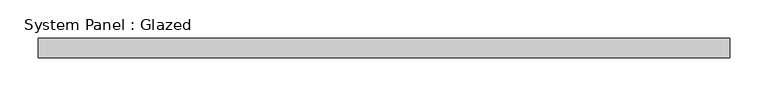
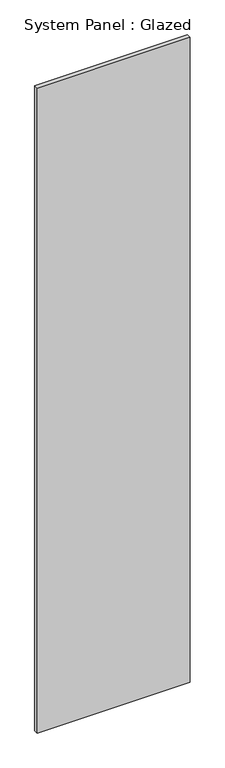
"""IFC4 building model written with IfcOpenShell, lengths in millimetres: plate geometry, System Panel : Glazed."""

from ifc_helpers import new_model, si_unit, origin, origin_with_axes, place, context, project, spatial, polyline, outline, extrude, source, transform, mapped, element, save


def system_panel_glazed_76c655e3(model_context):
    return source(origin(), model_context, "Body", "SweptSolid", [
        extrude(outline(polyline([(448.8630077, 24.5), (-448.8630077, 24.5), (-448.8630077, 49.5), (448.8630077, 49.5), (448.8630077, 24.5)])), origin_with_axes(), (0.0, 0.0, 1.0), 4000.0),
    ])


if __name__ == "__main__":
    model = new_model("IFC4")
    model_context = context("Model", 3, world=origin())
    ifc_project = project(units=[si_unit("LENGTHUNIT", "METRE", prefix="MILLI")], contexts=[model_context])
    site = spatial("IfcSite", under=ifc_project)
    building = spatial("IfcBuilding", under=site)
    placement = place(None, origin())
    system_panel_glazed_shape = system_panel_glazed_76c655e3(model_context)
    element("IfcPlate", 1, ObjectType="System Panel : Glazed", at=placement, inside=building, context=model_context, shape_type="MappedRepresentation", body=[
        mapped(system_panel_glazed_shape, transform((0.0, 0.0, 0.0), x_axis=(1.0, 0.0, 0.0), y_axis=(0.0, 1.0, 0.0), z_axis=(0.0, 0.0, 1.0))),
    ])
    save(model, "model.ifc")

# Revit data of these elements
# Type "System Panel : Glazed"
#   Keynote = "H11"
#   Construction Type Id = "GSP4R"
#   Analytic Construction = "1/8 in Pilkington single glazing"
#   Visual Light Transmittance = 0.9
#   Solar Heat Gain Coefficient = 0.86
#   Heat Transfer Coefficient (U) = 6.7069 W/(m²·K)
#   Define Thermal Properties by = 1
# Element 1 (IfcPlate, "System Panel : Glazed")
#   Materials on its faces: "Glass"
# Materials
#   "Glass": class "Glass", colour RGB 0 128 192, transparency 0.9, Description = "Soda Lime Glass", Cost = 0
